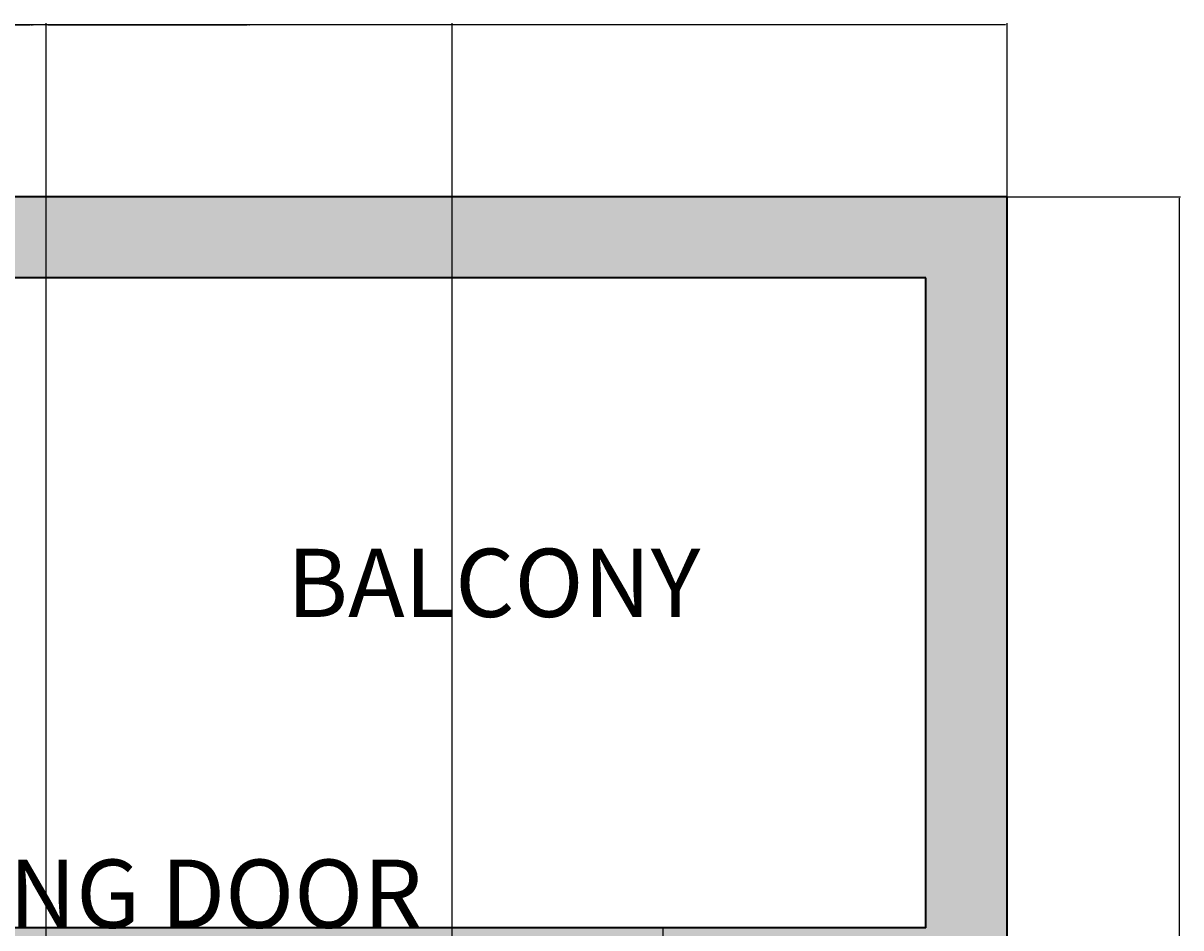
# Model space of a CAD drawing. Units: inches. Extents: x 857 to 1111, y 424 to 822.
# Tile 9 of 9: x 983 to 1111, y 722 to 822. Entities that reach past the tile are written whole.
import ezdxf

# ---------------------------------------------------------------- set-up
doc = ezdxf.new("R2010")
doc.units = ezdxf.units.IN
for name, color, linetype, lineweight in [('A-ANNO-DIMS', 2, 'Continuous', 18), ('A-ANNO-TEXT', 7, 'Continuous', 18), ('A-AREA-IDEN', 7, 'Continuous', 25), ('A-DOOR', 3, 'Continuous', 25), ('A-DOOR-PATT', 17, 'Continuous', 13), ('A-WALL', 7, 'Continuous', 35), ('A-WALL-PATT', 252, 'Continuous', 13)]:
    doc.layers.add(name, color=color, linetype=linetype, lineweight=lineweight)
doc.styles.get("Standard").update_dxf_attribs({"font": 'arial.ttf'})
doc.dimstyles.get("Standard").update_dxf_attribs({"dimtxt": 0.18, "dimasz": 0.18, "dimexe": 0.18, "dimexo": 0.0625, "dimgap": 0.09, "dimtad": 0, "dimtih": 1, "dimtoh": 1, "dimdec": 4, "dimzin": 0, "dimdsep": 46, "dimtxsty": 'Standard', "dimcen": 0.09, "dimadec": 0, "dimazin": 0, "dimtfac": 1, "dimtdec": 4, "dimtofl": 0, "dimtmove": 0, "dimatfit": 3, "dimfxl": 1, "dimtolj": 1, "dimtzin": 0, "dimarcsym": 0})

# ---------------------------------------------------------------- blocks, each defined once
blk = doc.blocks.new('*D44')
at = {"layer": 'A-ANNO-DIMS', "color": 0, "lineweight": -2, "transparency": 16777216}
for p, q in [((876.14, 802.92), (876.14, 822.09)), ((876.32, 821.91), (983.85, 821.91)), ((1091.96, 821.91), (984.43, 821.91)), ((1092.14, 802.92), (1092.14, 822.09))]:
    blk.add_line(p, q, dxfattribs=at)
at = {"layer": 'A-ANNO-DIMS', "color": 0, "transparency": 16777216}
for points in [[(876.32, 821.94), (876.32, 821.88), (876.14, 821.91)], [(1091.96, 821.94), (1091.96, 821.88), (1092.14, 821.91)]]:
    blk.add_solid(points, dxfattribs=at)
at = {"layer": 'Defpoints', "color": 0, "transparency": 16777216}
for p in [(1092.14, 821.91), (876.14, 802.86), (1092.14, 802.86)]:
    blk.add_point(p, dxfattribs=at)
at = {"layer": 'A-ANNO-DIMS', "color": 0, "transparency": 16777216, "insert": (984.14, 821.91), "char_height": 0.18, "attachment_point": 5}
blk.add_mtext('\\A1;216', dxfattribs=at)
blk = doc.blocks.new('*D45')
at = {"layer": 'A-ANNO-DIMS', "color": 0, "lineweight": -2, "transparency": 16777216}
for p, q in [((1092.2, 802.86), (1111.37, 802.86)), ((1111.19, 802.68), (1111.19, 623.04)), ((1111.19, 443.04), (1111.19, 622.67)), ((1092.2, 442.86), (1111.37, 442.86))]:
    blk.add_line(p, q, dxfattribs=at)
at = {"layer": 'A-ANNO-DIMS', "color": 0, "transparency": 16777216}
for points in [[(1111.16, 802.68), (1111.22, 802.68), (1111.19, 802.86)], [(1111.16, 443.04), (1111.22, 443.04), (1111.19, 442.86)]]:
    blk.add_solid(points, dxfattribs=at)
at = {"layer": 'Defpoints', "color": 0, "transparency": 16777216}
for p in [(1092.14, 802.86), (1111.19, 802.86), (1092.14, 442.86)]:
    blk.add_point(p, dxfattribs=at)
at = {"layer": 'A-ANNO-DIMS', "color": 0, "transparency": 16777216, "insert": (1111.19, 622.86), "char_height": 0.18, "attachment_point": 5}
blk.add_mtext('\\A1;360', dxfattribs=at)
blk = doc.blocks.new('*D48')
at = {"layer": 'A-ANNO-DIMS', "color": 0, "lineweight": -2, "transparency": 16777216}
for p, q in [((885.14, 582.42), (885.14, 822.09)), ((885.32, 821.91), (935, 821.91)), ((985.46, 821.91), (935.77, 821.91)), ((985.64, 582.42), (985.64, 822.09))]:
    blk.add_line(p, q, dxfattribs=at)
at = {"layer": 'A-ANNO-DIMS', "color": 0, "transparency": 16777216}
for points in [[(885.32, 821.94), (885.32, 821.88), (885.14, 821.91)], [(985.46, 821.94), (985.46, 821.88), (985.64, 821.91)]]:
    blk.add_solid(points, dxfattribs=at)
at = {"layer": 'Defpoints', "color": 0, "transparency": 16777216}
for p in [(985.64, 821.91), (885.14, 582.36), (985.64, 582.36)]:
    blk.add_point(p, dxfattribs=at)
at = {"layer": 'A-ANNO-DIMS', "color": 0, "transparency": 16777216, "insert": (935.39, 821.91), "char_height": 0.18, "attachment_point": 5}
blk.add_mtext('\\A1;100.5', dxfattribs=at)
blk = doc.blocks.new('*D49')
at = {"layer": 'A-ANNO-DIMS', "color": 0, "lineweight": -2, "transparency": 16777216}
for p, q in [((985.64, 451.92), (985.64, 822.09)), ((985.82, 821.91), (1007.91, 821.91)), ((1030.46, 821.91), (1008.36, 821.91)), ((1030.64, 451.92), (1030.64, 822.09))]:
    blk.add_line(p, q, dxfattribs=at)
at = {"layer": 'A-ANNO-DIMS', "color": 0, "transparency": 16777216}
for points in [[(985.82, 821.94), (985.82, 821.88), (985.64, 821.91)], [(1030.46, 821.94), (1030.46, 821.88), (1030.64, 821.91)]]:
    blk.add_solid(points, dxfattribs=at)
at = {"layer": 'Defpoints', "color": 0, "transparency": 16777216}
for p in [(1030.64, 821.91), (985.64, 451.86), (1030.64, 451.86)]:
    blk.add_point(p, dxfattribs=at)
at = {"layer": 'A-ANNO-DIMS', "color": 0, "transparency": 16777216, "insert": (1008.14, 821.91), "char_height": 0.18, "attachment_point": 5}
blk.add_mtext('\\A1;45', dxfattribs=at)

msp = doc.modelspace()

# ---------------------------------------------------------------- hatches: boundary and pattern name
at = {"layer": 'A-DOOR-PATT'}
h = msp.add_hatch(color=256, dxfattribs=at)
h.dxf.hatch_style = 1
h.set_gradient(color1=(0, 0, 255), color2=(255, 255, 0))
h.paths.add_polyline_path([(1053.9717, 718.9594), (969.1676, 718.9594), (969.1596, 718.4668), (927.0274, 718.4668), (924.7696, 718.4668), (924.7696, 717.3567), (1053.9717, 717.3567)], flags=17)
h.paths.add_polyline_path([(969.1676, 718.9594), (969.1922, 720.4869), (927.0274, 720.4869, -0.93409348), (927.0274, 718.4668), (969.1596, 718.4668)], flags=0)
h.paths.add_polyline_path([(1053.9717, 721.8567), (924.7696, 721.8567), (924.7696, 720.4869), (926.8896, 720.4869, -0.03407618), (927.0274, 720.4869), (927.0302, 720.4869), (969.1922, 720.4869), (969.1759, 719.4769), (1053.9717, 719.4769)], flags=17)
h.paths.add_polyline_path([(1053.9717, 721.8567), (924.7696, 721.8567), (924.7696, 717.3567), (1053.9717, 717.3567)])
h.paths.add_polyline_path([(969.1596, 718.4668), (927.0274, 718.4668, 0.93409348), (927.0274, 720.4869), (969.1922, 720.4869)], flags=16)
h = msp.add_hatch(color=256, dxfattribs=at)
h.dxf.hatch_style = 1
h.set_gradient(color1=(0, 0, 255), color2=(255, 255, 0), name='INVCYLINDER')
h.paths.add_polyline_path([(1053.9717, 721.8567), (924.7696, 721.8567), (924.7696, 720.4869), (927.0302, 720.4869), (969.1922, 720.4869), (969.1759, 719.4769), (1053.9717, 719.4769)], flags=17)
h.paths.add_polyline_path([(1053.9717, 718.9594), (969.1676, 718.9594), (969.1759, 719.4769), (1053.9717, 719.4769), (1053.9717, 721.8567), (924.7696, 721.8567), (924.7696, 717.3567), (1053.9717, 717.3567)])
h.paths.add_polyline_path([(969.1596, 718.4668), (927.0274, 718.4668, 0.93409348), (927.0274, 720.4869), (969.1922, 720.4869)], flags=16)
h = msp.add_hatch(color=256, dxfattribs=at)
h.dxf.hatch_style = 1
h.set_gradient(color1=(0, 0, 255), color2=(255, 255, 0), name='SPHERICAL')
h.paths.add_polyline_path([(1053.9717, 721.8567), (924.7696, 721.8567), (924.7696, 717.3567), (1053.9717, 717.3567), (1053.9717, 718.9594), (969.1676, 718.9594), (969.1759, 719.4769), (1053.9717, 719.4769)])
h.paths.add_polyline_path([(927.0274, 720.4869, -0.93409348), (927.0274, 718.4668), (969.1596, 718.4668), (969.1922, 720.4869)], flags=16)
at = {"layer": 'A-WALL-PATT'}
h = msp.add_hatch(color=256, dxfattribs=at)
h.dxf.hatch_style = 1
h.paths.add_polyline_path([(924.7696, 721.8567), (885.1369, 721.8567), (885.1369, 793.8567), (1083.1369, 793.8567), (1083.1369, 721.8567), (1053.9717, 721.8567), (1053.9717, 717.3567), (1083.1369, 717.3567), (1083.1369, 706.6069), (1092.1369, 706.6069), (1092.1369, 802.8567), (876.1369, 802.8567), (876.1369, 664.6868), (885.1369, 664.6868), (885.1369, 717.3567), (924.7696, 717.3567)])
h.paths.add_polyline_path([(985.6369, 582.3567), (885.1369, 582.3567), (885.1369, 585.1154), (885.1369, 628.6868), (876.1369, 628.6868), (876.1369, 529.0363), (885.1369, 529.0363), (885.1369, 577.8567), (981.1369, 577.8567), (985.6369, 577.8567)])
h.paths.add_polyline_path([(885.1369, 493.0363), (876.1369, 493.0363), (876.1369, 442.8567), (991.6369, 442.8567), (991.6369, 451.8567), (985.6369, 451.8567), (985.6369, 535.8567), (981.1369, 535.8567), (981.1369, 451.8567), (885.1369, 451.8567)])
h.paths.add_polyline_path([(1092.1369, 553.8025), (1083.1369, 553.8025), (1083.1369, 451.8567), (1030.6369, 451.8567), (1027.6369, 451.8567), (1027.6369, 442.8567), (1092.1369, 442.8567)])
h.paths.add_polyline_path([(1092.1369, 670.6069), (1083.1369, 670.6069), (1083.1369, 662.5384, -0.02676862), (1083.1369, 657.4501), (1083.1369, 589.8025), (1092.1369, 589.8025)])

# ---------------------------------------------------------------- linework, layer by layer
at = {"layer": 'A-DOOR'}
msp.add_lwpolyline([(924.7696, 721.8567), (1053.9717, 721.8567), (1053.9717, 717.3567), (924.7696, 717.3567)], close=True, dxfattribs=at)
at = {"layer": 'A-WALL'}
for p, q in [((1083.1369, 793.8567), (885.1369, 793.8567)), ((1083.1369, 721.8567), (1083.1369, 793.8567)), ((1083.1369, 721.8567), (885.1369, 721.8567))]:
    msp.add_line(p, q, dxfattribs=at)
msp.add_lwpolyline([(1027.6369, 442.8567), (1092.1369, 442.8567), (1092.1369, 802.8567), (876.1369, 802.8567), (876.1369, 442.8567), (991.6369, 442.8567)], dxfattribs=at)

# ---------------------------------------------------------------- texts
at = {"layer": 'A-ANNO-TEXT'}
msp.add_text('SLIDING DOOR ', height=7.55928, dxfattribs=at).set_placement((956.6211, 721.8567))
at = {"layer": 'A-AREA-IDEN'}
msp.add_text('BALCONY ', height=7.55928, dxfattribs=at).set_placement((1012.3237, 756.2969))

# ---------------------------------------------------------------- dimensions: what is measured, and where the dimension line sits
at = {"layer": 'A-ANNO-DIMS'}
for base, p1, p2, override, picture, middle in [((1092.1369, 821.9067), (876.1369, 802.8567), (1092.1369, 802.8567), {"dimdec": 0, "dimlfac": 1, "dimrnd": 0, "dimzin": 0, "dimdsep": 46, "dimlunit": 2}, '*D44', (984.1369, 821.9067)), ((985.6369, 821.9067), (885.1369, 582.3567), (985.6369, 582.3567), {"dimdec": 1, "dimlfac": 1, "dimrnd": 0, "dimzin": 0, "dimdsep": 46, "dimlunit": 2}, '*D48', (935.3869, 821.9067)), ((1030.6369, 821.9067), (985.6369, 451.8567), (1030.6369, 451.8567), {"dimdec": 0, "dimlfac": 1, "dimrnd": 0, "dimzin": 0, "dimdsep": 46, "dimlunit": 2}, '*D49', (1008.1369, 821.9067))]:
    dim = msp.add_linear_dim(base=base, p1=p1, p2=p2, dimstyle='Standard', override=override, dxfattribs=at)
    dim.commit()
    dim.dimension.update_dxf_attribs({"geometry": picture, "text_midpoint": middle})
dim = msp.add_linear_dim(base=(1111.1869, 802.8567), p1=(1092.1369, 442.8567), p2=(1092.1369, 802.8567), angle=90, dimstyle='Standard', override={"dimdec": 0, "dimlfac": 1, "dimrnd": 0, "dimzin": 0, "dimdsep": 46, "dimlunit": 2}, dxfattribs=at)
dim.commit()
dim.dimension.update_dxf_attribs({"geometry": '*D45', "text_midpoint": (1111.1869, 622.8567)})

doc.saveas('drawing.dxf')
